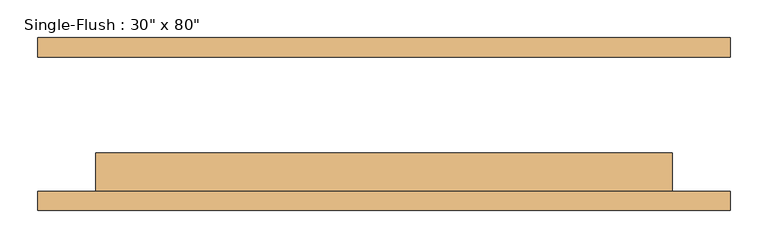
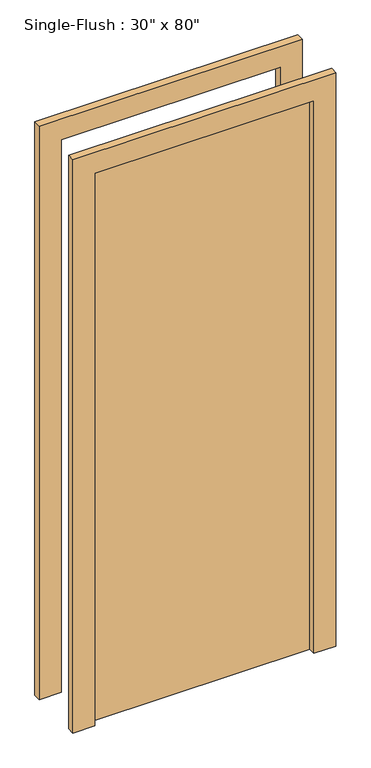
"""IFC4 building model written with IfcOpenShell, lengths in millimetres: door geometry."""

from ifc_helpers import new_model, si_unit, frame, origin, origin_with_axes, place, context, project, spatial, polyline, outline, extrude, source, transform, mapped, element, save


def door_ebd1a24e(model_context):
    return source(origin(), model_context, "Body", "SweptSolid", [
        extrude(outline(polyline([(2108.2, -457.2), (0.0, -457.2), (0.0, -381.0), (2032.0, -381.0), (2032.0, 381.0), (0.0, 381.0), (0.0, 457.2), (2108.2, 457.2), (2108.2, -457.2)])), frame((0.0, -114.3, 0.0), z_axis=(0.0, 1.0, 0.0), x_axis=(0.0, 0.0, 1.0)), (0.0, 0.0, 1.0), 25.4),
        extrude(outline(polyline([(2108.2, 457.2), (2108.2, -457.2), (0.0, -457.2), (0.0, -381.0), (2032.0, -381.0), (2032.0, 381.0), (0.0, 381.0), (0.0, 457.2), (2108.2, 457.2)])), frame((0.0, 88.9, 0.0), z_axis=(0.0, 1.0, 0.0), x_axis=(0.0, 0.0, 1.0)), (0.0, 0.0, 1.0), 25.4),
        extrude(outline(polyline([(381.0, -38.1), (381.0, -88.9), (-381.0, -88.9), (-381.0, -38.1), (381.0, -38.1)])), origin_with_axes(), (0.0, 0.0, 1.0), 2032.0),
    ])


if __name__ == "__main__":
    model = new_model("IFC4")
    model_context = context("Model", 3, world=origin())
    ifc_project = project(units=[si_unit("LENGTHUNIT", "METRE", prefix="MILLI")], contexts=[model_context])
    site = spatial("IfcSite", under=ifc_project)
    building = spatial("IfcBuilding", under=site)
    placement = place(None, origin())
    door_shape = door_ebd1a24e(model_context)
    element("IfcDoor", 1, ObjectType="Single-Flush : 30\" x 80\"", at=placement, inside=building, context=model_context, shape_type="MappedRepresentation", body=[
        mapped(door_shape, transform((0.0, 0.0, 0.0), x_axis=(1.0, 0.0, 0.0), y_axis=(0.0, 1.0, 0.0), z_axis=(0.0, 0.0, 1.0))),
    ])
    save(model, "model.ifc")

# Revit data of these elements
# Type "Single-Flush : 30\" x 80\""
#   Type Mark = "5"
#   Construction Type Id = "MDOOR"
#   Assembly Code = "C1020"
#   Analytic Construction = "Metal"
#   Thickness = 0' - 2"
#   Heat Transfer Coefficient (U) = 0.651978 BTU/(h·ft²·°F)
#   Height = 6' - 8"
#   Trim Projection Ext = 0' - 1"
#   Trim Projection Int = 0' - 1"
#   Trim Width = 0' - 3"
#   Width = 2' - 6"
#   Define Thermal Properties by = 1
#   Door Material = Door - Panel
#   Frame Material = Door - Frame
#   Visual Light Transmittance = 0
#   Solar Heat Gain Coefficient = 0
#   Function = (empty or 0)
#   Wall Closure = (empty or 0)
# Element 1 (IfcDoor, "Single-Flush : 30\" x 80\"")
#   Materials on its faces: "Door - Frame", "Door - Panel"
# Materials
#   "Door - Panel": class "Wood", colour RGB 210 159 95, transparency 0
#   "Door - Frame": colour RGB 118 70 51, transparency 0
